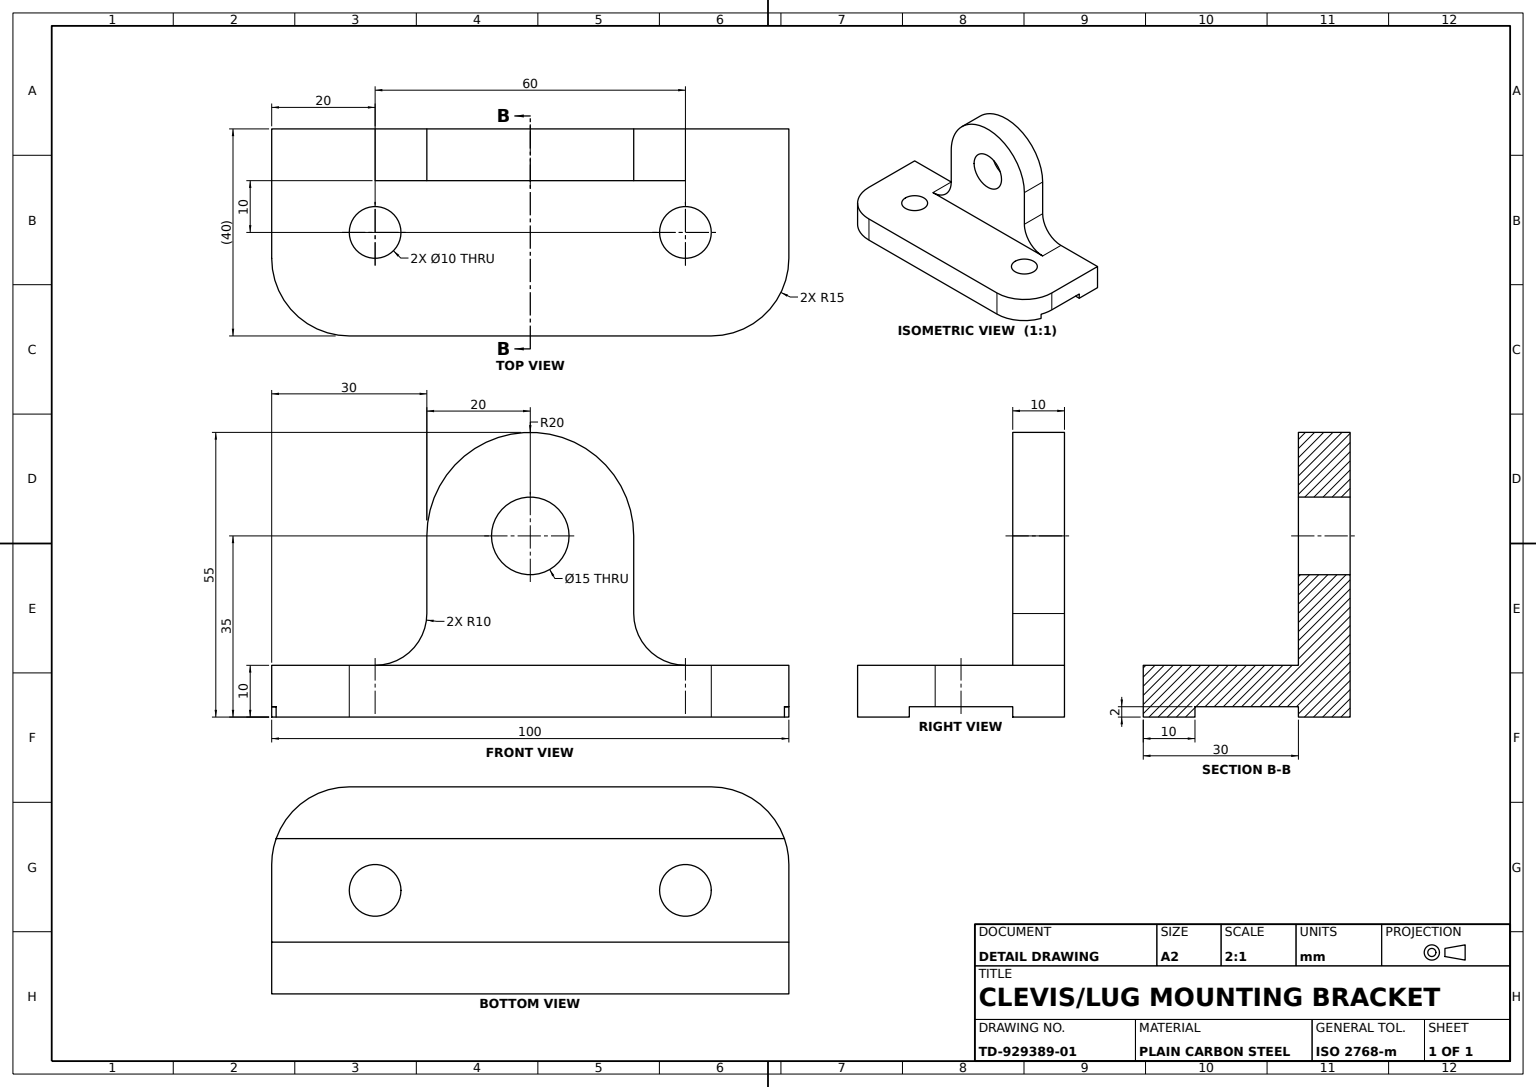
from build123d import *
from OCP.BRepFilletAPI import BRepFilletAPI_MakeFillet

# Parameters (mm, degrees)
BASE_AND_EAR_PROFILE_SKETCH_W       = 100
BASE_AND_EAR_PROFILE_SKETCH_H       = 10
BASE_PLATE_DEPTH                    = 40
SKETCH1_3_R                         = 20
SKETCH1_3_R_2                       = 7.5
CLEVIS_EAR_DEPTH                    = 10
MOUNTING_HOLES_2X_REACH             = 80.262
MOUNTING_HOLES_SKETCH_R             = 5
MOUNTING_HOLES_2X_DIRECTION_2_DEPTH = 79.262379212
CORNER_AND_EAR_FILLETS_R1           = 10
CORNER_AND_EAR_FILLETS_R2           = 15
BOTTOM_GROOVE_DEPTH                 = 85.409715081
BOTTOM_GROOVE_DEPTH_BACK            = 85.409715081
BOTTOM_GROOVE_SKETCH_W              = 20
BOTTOM_GROOVE_SKETCH_H              = 2


with BuildPart() as part:
    # Base and Ear Profile Sketch → Base Plate (new body)
    with BuildSketch(Plane.XY):
        with Locations((0, 5)):
            Rectangle(BASE_AND_EAR_PROFILE_SKETCH_W, BASE_AND_EAR_PROFILE_SKETCH_H)
    extrude(amount=BASE_PLATE_DEPTH)

    # Sketch1_3 → Clevis Ear (add)
    # profile 1 of 2: a face of its own
    with BuildSketch(Plane.XY):
        with BuildLine():
            Line((-20, 35), (-20, 10))
            Line((-20, 10), (20, 10))
            Line((20, 10), (20, 35))
            ThreePointArc((20, 35), (0, 15), (-20, 35))
        make_face()
    # profile 2 of 2: a face of its own
    with BuildSketch(Plane.XY):
        with Locations((0, 35)):
            Circle(SKETCH1_3_R)
        with Locations((0, 35)):
            Circle(SKETCH1_3_R_2, mode=Mode.SUBTRACT)
    extrude(amount=CLEVIS_EAR_DEPTH)

    # Mounting Holes Sketch → Mounting Holes 2x (cut, up to next)
    with BuildSketch(Plane(origin=(0, 10, 0), x_dir=(1, 0, 0), z_dir=(0, 1, 0)), mode=Mode.PRIVATE) as mounting_holes_2x_sk1:
        with Locations(Location((30, -20, 0), (0, 0, 180))):
            Circle(MOUNTING_HOLES_SKETCH_R)
    mounting_holes_2x_tool1 = extrude(mounting_holes_2x_sk1.sketch, amount=-MOUNTING_HOLES_2X_REACH, mode=Mode.PRIVATE) & part.part
    # Mounting Holes Sketch → Mounting Holes 2x (cut, up to next)
    with BuildSketch(Plane(origin=(0, 10, 0), x_dir=(1, 0, 0), z_dir=(0, 1, 0)), mode=Mode.PRIVATE) as mounting_holes_2x_sk2:
        with Locations(Location((-30, -20, 0), (0, 0, 180))):
            Circle(MOUNTING_HOLES_SKETCH_R)
    mounting_holes_2x_tool2 = extrude(mounting_holes_2x_sk2.sketch, amount=-MOUNTING_HOLES_2X_REACH, mode=Mode.PRIVATE) & part.part
    add(mounting_holes_2x_tool1.solids().sort_by_distance((30, 10, 20))[0], mode=Mode.SUBTRACT)
    add(mounting_holes_2x_tool2.solids().sort_by_distance((-30, 10, 20))[0], mode=Mode.SUBTRACT)

    # Mounting Holes Sketch → Mounting Holes 2x direction 2 (cut)
    with BuildSketch(Plane(origin=(0, 10, 0), x_dir=(1, 0, 0), z_dir=(0, 1, 0))):
        with Locations(Location((30, -20, 0), (0, 0, 180))):
            Circle(MOUNTING_HOLES_SKETCH_R)
        with Locations(Location((-30, -20, 0), (0, 0, 180))):
            Circle(MOUNTING_HOLES_SKETCH_R)
    extrude(amount=MOUNTING_HOLES_2X_DIRECTION_2_DEPTH, mode=Mode.SUBTRACT)

    # Corner and Ear Fillets: one fillet with a radius per group of edges: ONE call of the kernel's fillet builder (fillet() takes one radius for all edges)
    corner_and_ear_fillets_edges_1 = [part.edges().sort_by_distance(p)[0] for p in [
        (20, 10, 5),
        (-20, 10, 5),
    ]]
    corner_and_ear_fillets_edges_2 = [part.edges().sort_by_distance(p)[0] for p in [
        (-50, 5, 40),
        (50, 5, 40),
    ]]
    corner_and_ear_fillets = BRepFilletAPI_MakeFillet(part.part.solid().wrapped)
    for e in corner_and_ear_fillets_edges_1:
        corner_and_ear_fillets.Add(CORNER_AND_EAR_FILLETS_R1, e.wrapped)
    for e in corner_and_ear_fillets_edges_2:
        corner_and_ear_fillets.Add(CORNER_AND_EAR_FILLETS_R2, e.wrapped)
    add(Compound.cast(corner_and_ear_fillets.Shape()), mode=Mode.REPLACE)

    # Bottom Groove Sketch → Bottom Groove (cut, two sides: drawn at the far end of the back side and taken through both)
    with BuildSketch(Plane(origin=(0, 0, 0), x_dir=(0, 0, -1), z_dir=(1, 0, 0)).offset(-BOTTOM_GROOVE_DEPTH_BACK)):
        with Locations((-20, 1)):
            Rectangle(BOTTOM_GROOVE_SKETCH_W, BOTTOM_GROOVE_SKETCH_H)
    extrude(amount=BOTTOM_GROOVE_DEPTH + BOTTOM_GROOVE_DEPTH_BACK, mode=Mode.SUBTRACT)


solid = part.part
